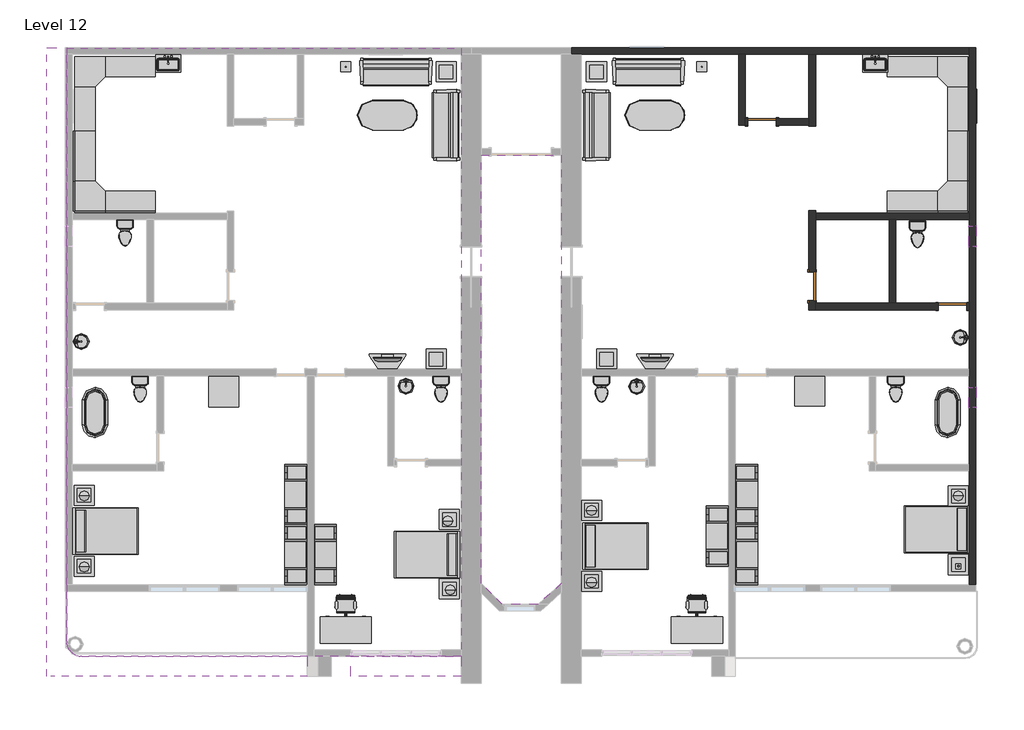
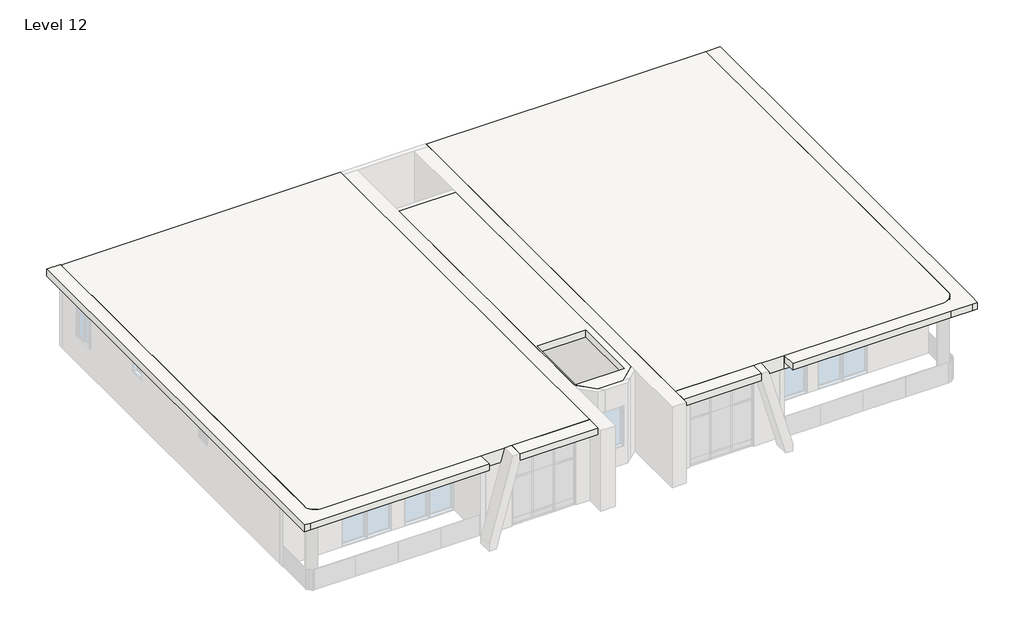
# One storey, part 3 of 3: 42 furniture elements, 14 flow terminals, 10 light fixtures, 9 walls, 4 slabs, 3 doors, 3 windows.
"""IFC4 building model written with IfcOpenShell, lengths in millimetres."""

from ifc_helpers import new_model, si_unit, point, frame, frame_2d, origin, place, context, project, spatial, polyline, circle_curve, trimmed, segment, composite_curve, outline, extrude, faceted_brep, transform, mapped, element, save
from components import door_2703ae13, door_10fd3a06, flow_terminal_38af2918, flow_terminal_d49f872f, toilet_domestic_3d_toilet_domestic_3d_f7549cf7, toilet_domestic_3d_toilet_domestic_3d_183bbd19, flow_terminal_b374fae2, furniture_07436f11, furniture_096e7f55, chair_task_arms_chair_task_arms_fa5a08ef, furniture_072f6425, furniture_cf0b6580, furniture_aff9b2fb, furniture_56245f3a, tv_stand_tv_stand_6ce107e5, furniture_b5c51a22, furniture_2c34a4f9, furniture_4d44e21c, furniture_45e3acac, light_fixture_100w_120v_8564026f, table_lamp_hemispheric_60w_120v_02721d88, window_0038ecf3, window_54100e87

model = new_model("IFC4")

# Units and contexts
model_context = context("Model", 3, world=origin())
ifc_project = project(units=[si_unit("LENGTHUNIT", "METRE", prefix="MILLI")], contexts=[model_context])

# Site, building, storey
site = spatial("IfcSite", under=ifc_project)
building = spatial("IfcBuilding", under=site)
storey = spatial("IfcBuildingStorey", under=building, Name="Level 12", Elevation=40233.6)

# Doors
placement = place(None, origin())
door_shape = door_2703ae13(model_context)
element("IfcDoor", 1, ObjectType="Door-Single-Panel.0001 : 34\" x 80\"", at=placement, inside=storey, context=model_context, shape_type="MappedRepresentation", body=[
    mapped(door_shape, transform((2522.0012296, 9464.0758558, 40233.6), x_axis=(-1.0, 0.0, 0.0), y_axis=(0.0, -1.0, 0.0), z_axis=(0.0, 0.0, 1.0))),
])
door_2_shape = door_10fd3a06(model_context)
element("IfcDoor", 2, ObjectType="Door-Single-Panel.0001 : 34\" x 80\"", at=placement, inside=storey, context=model_context, shape_type="MappedRepresentation", body=[
    mapped(door_2_shape, transform((8313.2012296, 3850.6758558, 40233.6), x_axis=(1.0, 0.0, 0.0), y_axis=(0.0, 1.0, 0.0), z_axis=(0.0, 0.0, 1.0))),
])
element("IfcDoor", 3, ObjectType="Door-Single-Panel.0001 : 34\" x 80\"", at=placement, inside=storey, context=model_context, shape_type="MappedRepresentation", body=[
    mapped(door_2_shape, transform((4046.0012296, 4460.2758558, 40233.6), x_axis=(0.0, -1.0, 0.0), y_axis=(1.0, 0.0, 0.0), z_axis=(0.0, 0.0, 1.0))),
])

# Flow terminals
flow_terminal_shape = flow_terminal_38af2918(model_context)
element("IfcFlowTerminal", 4, ObjectType="Sink Kitchen-Single : 30\" x 21\"", at=placement, inside=storey, context=model_context, shape_type="MappedRepresentation", body=[
    mapped(flow_terminal_shape, transform((-15540.388011, 11239.7304546, 40233.6), x_axis=(1.0, 0.0, 0.0), y_axis=(0.0, 1.0, 0.0), z_axis=(0.0, 0.0, 1.0))),
])
element("IfcFlowTerminal", 5, ObjectType="Sink Kitchen-Single : 30\" x 21\"", at=placement, inside=storey, context=model_context, shape_type="MappedRepresentation", body=[
    mapped(flow_terminal_shape, transform((5948.011989, 11239.7304546, 40233.6), x_axis=(1.0, 0.0, 0.0), y_axis=(0.0, 1.0, 0.0), z_axis=(0.0, 0.0, 1.0))),
])
flow_terminal_2_shape = flow_terminal_d49f872f(model_context)
element("IfcFlowTerminal", 6, ObjectType="Sink Vanity-Round : 19\" x 19\"", at=placement, inside=storey, context=model_context, shape_type="MappedRepresentation", body=[
    mapped(flow_terminal_2_shape, transform((-18084.6070794, 2687.2241152, 40233.6), x_axis=(0.0, 1.0, 0.0), y_axis=(-1.0, 0.0, 0.0), z_axis=(0.0, 0.0, 1.0))),
])
element("IfcFlowTerminal", 7, ObjectType="Sink Vanity-Round : 19\" x 19\"", at=placement, inside=storey, context=model_context, shape_type="MappedRepresentation", body=[
    mapped(flow_terminal_2_shape, transform((8462.2249463, 3007.5275963, 40233.6), x_axis=(0.0, -1.0, 0.0), y_axis=(1.0, 0.0, 0.0), z_axis=(0.0, 0.0, 1.0))),
])
element("IfcFlowTerminal", 8, ObjectType="Sink Vanity-Round : 19\" x 19\"", at=placement, inside=storey, context=model_context, shape_type="MappedRepresentation", body=[
    mapped(flow_terminal_2_shape, transform((-8395.050511, 1341.8921141, 40233.6), x_axis=(1.0, 0.0, 0.0), y_axis=(0.0, 1.0, 0.0), z_axis=(0.0, 0.0, 1.0))),
])
element("IfcFlowTerminal", 9, ObjectType="Sink Vanity-Round : 19\" x 19\"", at=placement, inside=storey, context=model_context, shape_type="MappedRepresentation", body=[
    mapped(flow_terminal_2_shape, transform((-1384.650511, 1331.0855344, 40233.6), x_axis=(1.0, 0.0, 0.0), y_axis=(0.0, 1.0, 0.0), z_axis=(0.0, 0.0, 1.0))),
])
toilet_domestic_3d_toilet_domestic_3d_shape = toilet_domestic_3d_toilet_domestic_3d_f7549cf7(model_context)
toilet_domestic_3d_toilet_domestic_3d_2_shape = toilet_domestic_3d_toilet_domestic_3d_183bbd19(model_context)
element("IfcFlowTerminal", 10, ObjectType="Toilet-Domestic-3D : Toilet-Domestic-3D", at=placement, inside=storey, context=model_context, shape_type="MappedRepresentation", body=[
    mapped(toilet_domestic_3d_toilet_domestic_3d_shape, transform((6586.0012296, 1247.7798284, 40233.6), x_axis=(1.0, 0.0, 0.0), y_axis=(0.0, 1.0, 0.0), z_axis=(0.0, 0.0, 1.0))),
    mapped(toilet_domestic_3d_toilet_domestic_3d_2_shape, transform((6586.0012296, 1247.7798284, 40233.6), x_axis=(1.0, 0.0, 0.0), y_axis=(0.0, 1.0, 0.0), z_axis=(0.0, 0.0, 1.0))),
])
element("IfcFlowTerminal", 11, ObjectType="Toilet-Domestic-3D : Toilet-Domestic-3D", at=placement, inside=storey, context=model_context, shape_type="MappedRepresentation", body=[
    mapped(toilet_domestic_3d_toilet_domestic_3d_shape, transform((-2354.7987704, 1247.7798284, 40233.6), x_axis=(1.0, 0.0, 0.0), y_axis=(0.0, 1.0, 0.0), z_axis=(0.0, 0.0, 1.0))),
    mapped(toilet_domestic_3d_toilet_domestic_3d_2_shape, transform((-2354.7987704, 1247.7798284, 40233.6), x_axis=(1.0, 0.0, 0.0), y_axis=(0.0, 1.0, 0.0), z_axis=(0.0, 0.0, 1.0))),
])
element("IfcFlowTerminal", 12, ObjectType="Toilet-Domestic-3D : Toilet-Domestic-3D", at=placement, inside=storey, context=model_context, shape_type="MappedRepresentation", body=[
    mapped(toilet_domestic_3d_toilet_domestic_3d_shape, transform((-16375.5987704, 1247.7798284, 40233.6), x_axis=(1.0, 0.0, 0.0), y_axis=(0.0, 1.0, 0.0), z_axis=(0.0, 0.0, 1.0))),
    mapped(toilet_domestic_3d_toilet_domestic_3d_2_shape, transform((-16375.5987704, 1247.7798284, 40233.6), x_axis=(1.0, 0.0, 0.0), y_axis=(0.0, 1.0, 0.0), z_axis=(0.0, 0.0, 1.0))),
])
element("IfcFlowTerminal", 13, ObjectType="Toilet-Domestic-3D : Toilet-Domestic-3D", at=placement, inside=storey, context=model_context, shape_type="MappedRepresentation", body=[
    mapped(toilet_domestic_3d_toilet_domestic_3d_shape, transform((-16832.7987704, 5997.5798284, 40233.6), x_axis=(1.0, 0.0, 0.0), y_axis=(0.0, 1.0, 0.0), z_axis=(0.0, 0.0, 1.0))),
    mapped(toilet_domestic_3d_toilet_domestic_3d_2_shape, transform((-16832.7987704, 5997.5798284, 40233.6), x_axis=(1.0, 0.0, 0.0), y_axis=(0.0, 1.0, 0.0), z_axis=(0.0, 0.0, 1.0))),
])
element("IfcFlowTerminal", 14, ObjectType="Toilet-Domestic-3D : Toilet-Domestic-3D", at=placement, inside=storey, context=model_context, shape_type="MappedRepresentation", body=[
    mapped(toilet_domestic_3d_toilet_domestic_3d_shape, transform((7246.4012296, 5946.7798284, 40233.6), x_axis=(1.0, 0.0, 0.0), y_axis=(0.0, 1.0, 0.0), z_axis=(0.0, 0.0, 1.0))),
    mapped(toilet_domestic_3d_toilet_domestic_3d_2_shape, transform((7246.4012296, 5946.7798284, 40233.6), x_axis=(1.0, 0.0, 0.0), y_axis=(0.0, 1.0, 0.0), z_axis=(0.0, 0.0, 1.0))),
])
element("IfcFlowTerminal", 15, ObjectType="Toilet-Domestic-3D : Toilet-Domestic-3D", at=placement, inside=storey, context=model_context, shape_type="MappedRepresentation", body=[
    mapped(toilet_domestic_3d_toilet_domestic_3d_shape, transform((-7231.5987704, 1247.7798284, 40233.6), x_axis=(1.0, 0.0, 0.0), y_axis=(0.0, 1.0, 0.0), z_axis=(0.0, 0.0, 1.0))),
    mapped(toilet_domestic_3d_toilet_domestic_3d_2_shape, transform((-7231.5987704, 1247.7798284, 40233.6), x_axis=(1.0, 0.0, 0.0), y_axis=(0.0, 1.0, 0.0), z_axis=(0.0, 0.0, 1.0))),
])
flow_terminal_3_shape = flow_terminal_b374fae2(model_context)
element("IfcFlowTerminal", 16, ObjectType="Tub-Free Standing-3D : 30\" x 60\"", at=placement, inside=storey, context=model_context, shape_type="MappedRepresentation", body=[
    mapped(flow_terminal_3_shape, transform((-17747.1987704, 624.8758558, 40233.6), x_axis=(1.0, 0.0, 0.0), y_axis=(0.0, 1.0, 0.0), z_axis=(0.0, 0.0, 1.0))),
])
element("IfcFlowTerminal", 17, ObjectType="Tub-Free Standing-3D : 30\" x 60\"", at=placement, inside=storey, context=model_context, shape_type="MappedRepresentation", body=[
    mapped(flow_terminal_3_shape, transform((8160.8012296, 624.8758558, 40233.6), x_axis=(1.0, 0.0, 0.0), y_axis=(0.0, 1.0, 0.0), z_axis=(0.0, 0.0, 1.0))),
])

# Furniture
furniture_shape = furniture_07436f11(model_context)
element("IfcFurniture", 18, ObjectType="96\" x 96\"", at=placement, inside=storey, context=model_context, shape_type="MappedRepresentation", body=[
    mapped(furniture_shape, transform((-18275.8670182, 11991.0988634, 40233.6), x_axis=(1.0, 0.0, 0.0), y_axis=(0.0, 1.0, 0.0), z_axis=(0.0, 0.0, 1.0))),
])
element("IfcFurniture", 19, ObjectType="96\" x 96\"", at=placement, inside=storey, context=model_context, shape_type="MappedRepresentation", body=[
    mapped(furniture_shape, transform((9316.2242372, 11364.3441035, 40233.6), x_axis=(0.0, -1.0, 0.0), y_axis=(1.0, 0.0, 0.0), z_axis=(0.0, 0.0, 1.0))),
])
furniture_2_shape = furniture_096e7f55(model_context)
element("IfcFurniture", 20, ObjectType="Bed-Shaker : Double 56\" x 78\"", at=placement, inside=storey, context=model_context, shape_type="MappedRepresentation", body=[
    mapped(furniture_2_shape, transform((-18407.5987704, -2962.8741442, 40233.6), x_axis=(0.0, 1.0, 0.0), y_axis=(-1.0, 0.0, 0.0), z_axis=(0.0, 0.0, 1.0))),
])
element("IfcFurniture", 21, ObjectType="Bed-Shaker : Double 56\" x 78\"", at=placement, inside=storey, context=model_context, shape_type="MappedRepresentation", body=[
    mapped(furniture_2_shape, transform((-6672.7987704, -3712.1741442, 40233.6), x_axis=(0.0, -1.0, 0.0), y_axis=(1.0, 0.0, 0.0), z_axis=(0.0, 0.0, 1.0))),
])
element("IfcFurniture", 22, ObjectType="Bed-Shaker : Double 56\" x 78\"", at=placement, inside=storey, context=model_context, shape_type="MappedRepresentation", body=[
    mapped(furniture_2_shape, transform((-2913.5987704, -3420.0741442, 40233.6), x_axis=(0.0, 1.0, 0.0), y_axis=(-1.0, 0.0, 0.0), z_axis=(0.0, 0.0, 1.0))),
])
element("IfcFurniture", 23, ObjectType="Bed-Shaker : Double 56\" x 78\"", at=placement, inside=storey, context=model_context, shape_type="MappedRepresentation", body=[
    mapped(furniture_2_shape, transform((8821.2012296, -2950.1741442, 40233.6), x_axis=(0.0, -1.0, 0.0), y_axis=(1.0, 0.0, 0.0), z_axis=(0.0, 0.0, 1.0))),
])
chair_task_arms_chair_task_arms_shape = chair_task_arms_chair_task_arms_fa5a08ef(model_context)
element("IfcFurniture", 24, ObjectType="Chair-Task Arms : Chair-Task Arms", at=placement, inside=storey, context=model_context, shape_type="MappedRepresentation", body=[
    mapped(chair_task_arms_chair_task_arms_shape, transform((681.7920493, -5184.3566833, 40233.6), x_axis=(-1.0, 0.0, 0.0), y_axis=(0.0, -1.0, 0.0), z_axis=(0.0, 0.0, 1.0))),
])
element("IfcFurniture", 25, ObjectType="Chair-Task Arms : Chair-Task Arms", at=placement, inside=storey, context=model_context, shape_type="MappedRepresentation", body=[
    mapped(chair_task_arms_chair_task_arms_shape, transform((-9986.2079507, -5184.3566833, 40233.6), x_axis=(-1.0, 0.0, 0.0), y_axis=(0.0, -1.0, 0.0), z_axis=(0.0, 0.0, 1.0))),
])
furniture_3_shape = furniture_072f6425(model_context)
element("IfcFurniture", 26, ObjectType="Desk : 60\" x 30\"", at=placement, inside=storey, context=model_context, shape_type="MappedRepresentation", body=[
    mapped(furniture_3_shape, transform((-10889.1987704, -6371.702585, 40233.6), x_axis=(1.0, 0.0, 0.0), y_axis=(0.0, 1.0, 0.0), z_axis=(0.0, 0.0, 1.0))),
])
element("IfcFurniture", 27, ObjectType="Desk : 60\" x 30\"", at=placement, inside=storey, context=model_context, shape_type="MappedRepresentation", body=[
    mapped(furniture_3_shape, transform((-221.1987704, -6371.702585, 40233.6), x_axis=(1.0, 0.0, 0.0), y_axis=(0.0, 1.0, 0.0), z_axis=(0.0, 0.0, 1.0))),
])
furniture_4_shape = furniture_cf0b6580(model_context)
element("IfcFurniture", 28, ObjectType="Entertainment Center : 72\" x 72\" x 24\"", at=placement, inside=storey, context=model_context, shape_type="MappedRepresentation", body=[
    mapped(furniture_4_shape, transform((1607.6012296, -3134.3241442, 40233.6), x_axis=(0.0, -1.0, 0.0), y_axis=(1.0, 0.0, 0.0), z_axis=(0.0, 0.0, 1.0))),
])
element("IfcFurniture", 29, ObjectType="Entertainment Center : 72\" x 72\" x 24\"", at=placement, inside=storey, context=model_context, shape_type="MappedRepresentation", body=[
    mapped(furniture_4_shape, transform((1607.6012296, -3693.1241442, 40233.6), x_axis=(0.0, 1.0, 0.0), y_axis=(-1.0, 0.0, 0.0), z_axis=(0.0, 0.0, 1.0))),
])
element("IfcFurniture", 30, ObjectType="Entertainment Center : 72\" x 72\" x 24\"", at=placement, inside=storey, context=model_context, shape_type="MappedRepresentation", body=[
    mapped(furniture_4_shape, transform((1607.6012296, -1864.3241442, 40233.6), x_axis=(0.0, 1.0, 0.0), y_axis=(-1.0, 0.0, 0.0), z_axis=(0.0, 0.0, 1.0))),
])
element("IfcFurniture", 31, ObjectType="Entertainment Center : 72\" x 72\" x 24\"", at=placement, inside=storey, context=model_context, shape_type="MappedRepresentation", body=[
    mapped(furniture_4_shape, transform((-11193.9987704, -3693.1241442, 40233.6), x_axis=(0.0, -1.0, 0.0), y_axis=(1.0, 0.0, 0.0), z_axis=(0.0, 0.0, 1.0))),
])
element("IfcFurniture", 32, ObjectType="Entertainment Center : 72\" x 72\" x 24\"", at=placement, inside=storey, context=model_context, shape_type="MappedRepresentation", body=[
    mapped(furniture_4_shape, transform((-11193.9987704, -1864.3241442, 40233.6), x_axis=(0.0, -1.0, 0.0), y_axis=(1.0, 0.0, 0.0), z_axis=(0.0, 0.0, 1.0))),
])
element("IfcFurniture", 33, ObjectType="Entertainment Center : 72\" x 72\" x 24\"", at=placement, inside=storey, context=model_context, shape_type="MappedRepresentation", body=[
    mapped(furniture_4_shape, transform((-11193.9987704, -3693.1241442, 40233.6), x_axis=(0.0, 1.0, 0.0), y_axis=(-1.0, 0.0, 0.0), z_axis=(0.0, 0.0, 1.0))),
])
furniture_5_shape = furniture_aff9b2fb(model_context)
element("IfcFurniture", 34, ObjectType="Sofa-Pensi : 84\"", at=placement, inside=storey, context=model_context, shape_type="MappedRepresentation", body=[
    mapped(furniture_5_shape, transform((-8881.8050204, 10710.9660197, 40233.6), x_axis=(1.0, 0.0, 0.0), y_axis=(0.0, 1.0, 0.0), z_axis=(0.0, 0.0, 1.0))),
])
element("IfcFurniture", 35, ObjectType="Sofa-Pensi : 84\"", at=placement, inside=storey, context=model_context, shape_type="MappedRepresentation", body=[
    mapped(furniture_5_shape, transform((-7356.3086065, 9641.0821058, 40233.6), x_axis=(0.0, -1.0, 0.0), y_axis=(1.0, 0.0, 0.0), z_axis=(0.0, 0.0, 1.0))),
])
element("IfcFurniture", 36, ObjectType="Sofa-Pensi : 84\"", at=placement, inside=storey, context=model_context, shape_type="MappedRepresentation", body=[
    mapped(furniture_5_shape, transform((-2230.0889343, 9083.8696058, 40233.6), x_axis=(0.0, 1.0, 0.0), y_axis=(-1.0, 0.0, 0.0), z_axis=(0.0, 0.0, 1.0))),
])
element("IfcFurniture", 37, ObjectType="Sofa-Pensi : 84\"", at=placement, inside=storey, context=model_context, shape_type="MappedRepresentation", body=[
    mapped(furniture_5_shape, transform((-1211.0050204, 10710.9660197, 40233.6), x_axis=(1.0, 0.0, 0.0), y_axis=(0.0, 1.0, 0.0), z_axis=(0.0, 0.0, 1.0))),
])
furniture_6_shape = furniture_56245f3a(model_context)
element("IfcFurniture", 38, ObjectType="TV - Flat Screen : 32\"", at=placement, inside=storey, context=model_context, shape_type="MappedRepresentation", body=[
    mapped(furniture_6_shape, transform((-8861.1432846, 2232.8144794, 41148.0), x_axis=(-1.0, 0.0, 0.0), y_axis=(0.0, -1.0, 0.0), z_axis=(0.0, 0.0, 1.0))),
])
element("IfcFurniture", 39, ObjectType="TV - Flat Screen : 32\"", at=placement, inside=storey, context=model_context, shape_type="MappedRepresentation", body=[
    mapped(furniture_6_shape, transform((-733.1432846, 2232.8144794, 41148.0), x_axis=(-1.0, 0.0, 0.0), y_axis=(0.0, -1.0, 0.0), z_axis=(0.0, 0.0, 1.0))),
])
tv_stand_tv_stand_shape = tv_stand_tv_stand_6ce107e5(model_context)
element("IfcFurniture", 40, ObjectType="TV Stand : TV Stand", at=placement, inside=storey, context=model_context, shape_type="MappedRepresentation", body=[
    mapped(tv_stand_tv_stand_shape, transform((-8732.0107683, 1945.6758558, 40233.6), x_axis=(-1.0, 0.0, 0.0), y_axis=(0.0, -1.0, 0.0), z_axis=(0.0, 0.0, 1.0))),
])
element("IfcFurniture", 41, ObjectType="TV Stand : TV Stand", at=placement, inside=storey, context=model_context, shape_type="MappedRepresentation", body=[
    mapped(tv_stand_tv_stand_shape, transform((-604.0107683, 1945.6758558, 40233.6), x_axis=(-1.0, 0.0, 0.0), y_axis=(0.0, -1.0, 0.0), z_axis=(0.0, 0.0, 1.0))),
])
furniture_7_shape = furniture_b5c51a22(model_context)
element("IfcFurniture", 42, ObjectType="Table-Coffee : 24\" x 24\" x 24\"", at=placement, inside=storey, context=model_context, shape_type="MappedRepresentation", body=[
    mapped(furniture_7_shape, transform((-7097.4645371, 10892.864778, 40233.6), x_axis=(1.0, 0.0, 0.0), y_axis=(0.0, 1.0, 0.0), z_axis=(0.0, 0.0, 1.0))),
])
element("IfcFurniture", 43, ObjectType="Table-Coffee : 24\" x 24\" x 24\"", at=placement, inside=storey, context=model_context, shape_type="MappedRepresentation", body=[
    mapped(furniture_7_shape, transform((-2525.4645371, 10892.864778, 40233.6), x_axis=(1.0, 0.0, 0.0), y_axis=(0.0, 1.0, 0.0), z_axis=(0.0, 0.0, 1.0))),
])
element("IfcFurniture", 44, ObjectType="Table-Coffee : 24\" x 24\" x 24\"", at=placement, inside=storey, context=model_context, shape_type="MappedRepresentation", body=[
    mapped(furniture_7_shape, transform((-7402.2645371, 2155.264778, 40233.6), x_axis=(1.0, 0.0, 0.0), y_axis=(0.0, 1.0, 0.0), z_axis=(0.0, 0.0, 1.0))),
])
element("IfcFurniture", 45, ObjectType="Table-Coffee : 24\" x 24\" x 24\"", at=placement, inside=storey, context=model_context, shape_type="MappedRepresentation", body=[
    mapped(furniture_7_shape, transform((-2220.6645371, 2155.264778, 40233.6), x_axis=(1.0, 0.0, 0.0), y_axis=(0.0, 1.0, 0.0), z_axis=(0.0, 0.0, 1.0))),
])
element("IfcFurniture", 46, ObjectType="Table-Coffee : 24\" x 24\" x 24\"", at=placement, inside=storey, context=model_context, shape_type="MappedRepresentation", body=[
    mapped(furniture_7_shape, transform((-2677.8645371, -4601.135222, 40233.6), x_axis=(1.0, 0.0, 0.0), y_axis=(0.0, 1.0, 0.0), z_axis=(0.0, 0.0, 1.0))),
])
element("IfcFurniture", 47, ObjectType="Table-Coffee : 24\" x 24\" x 24\"", at=placement, inside=storey, context=model_context, shape_type="MappedRepresentation", body=[
    mapped(furniture_7_shape, transform((-18095.6645371, -4143.935222, 40233.6), x_axis=(1.0, 0.0, 0.0), y_axis=(0.0, 1.0, 0.0), z_axis=(0.0, 0.0, 1.0))),
])
element("IfcFurniture", 48, ObjectType="Table-Coffee : 24\" x 24\" x 24\"", at=placement, inside=storey, context=model_context, shape_type="MappedRepresentation", body=[
    mapped(furniture_7_shape, transform((-18095.6645371, -1984.935222, 40233.6), x_axis=(1.0, 0.0, 0.0), y_axis=(0.0, 1.0, 0.0), z_axis=(0.0, 0.0, 1.0))),
])
element("IfcFurniture", 49, ObjectType="Table-Coffee : 24\" x 24\" x 24\"", at=placement, inside=storey, context=model_context, shape_type="MappedRepresentation", body=[
    mapped(furniture_7_shape, transform((-2677.8645371, -2442.135222, 40233.6), x_axis=(1.0, 0.0, 0.0), y_axis=(0.0, 1.0, 0.0), z_axis=(0.0, 0.0, 1.0))),
])
element("IfcFurniture", 50, ObjectType="Table-Coffee : 24\" x 24\" x 24\"", at=placement, inside=storey, context=model_context, shape_type="MappedRepresentation", body=[
    mapped(furniture_7_shape, transform((8472.7354629, -4093.135222, 40233.6), x_axis=(1.0, 0.0, 0.0), y_axis=(0.0, 1.0, 0.0), z_axis=(0.0, 0.0, 1.0))),
])
element("IfcFurniture", 51, ObjectType="Table-Coffee : 24\" x 24\" x 24\"", at=placement, inside=storey, context=model_context, shape_type="MappedRepresentation", body=[
    mapped(furniture_7_shape, transform((8472.7354629, -2010.335222, 40233.6), x_axis=(1.0, 0.0, 0.0), y_axis=(0.0, 1.0, 0.0), z_axis=(0.0, 0.0, 1.0))),
])
element("IfcFurniture", 52, ObjectType="Table-Coffee : 24\" x 24\" x 24\"", at=placement, inside=storey, context=model_context, shape_type="MappedRepresentation", body=[
    mapped(furniture_7_shape, transform((-6995.8645371, -4832.0414601, 40233.6), x_axis=(1.0, 0.0, 0.0), y_axis=(0.0, 1.0, 0.0), z_axis=(0.0, 0.0, 1.0))),
])
element("IfcFurniture", 53, ObjectType="Table-Coffee : 24\" x 24\" x 24\"", at=placement, inside=storey, context=model_context, shape_type="MappedRepresentation", body=[
    mapped(furniture_7_shape, transform((-6995.8645371, -2723.8414601, 40233.6), x_axis=(1.0, 0.0, 0.0), y_axis=(0.0, 1.0, 0.0), z_axis=(0.0, 0.0, 1.0))),
])
furniture_8_shape = furniture_2c34a4f9(model_context)
element("IfcFurniture", 54, ObjectType="Table-Dining Oval : 36\" x 72\"", at=placement, inside=storey, context=model_context, shape_type="MappedRepresentation", body=[
    mapped(furniture_8_shape, transform((-8455.3790983, 10025.3742164, 40233.6), x_axis=(1.0, 0.0, 0.0), y_axis=(0.0, 1.0, 0.0), z_axis=(0.0, 0.0, 1.0))),
])
element("IfcFurniture", 55, ObjectType="Table-Dining Oval : 36\" x 72\"", at=placement, inside=storey, context=model_context, shape_type="MappedRepresentation", body=[
    mapped(furniture_8_shape, transform((-327.3790983, 10025.3742164, 40233.6), x_axis=(1.0, 0.0, 0.0), y_axis=(0.0, 1.0, 0.0), z_axis=(0.0, 0.0, 1.0))),
])
furniture_9_shape = furniture_4d44e21c(model_context)
element("IfcFurniture", 56, ObjectType="Table-Rectangular : 36\" x 36\"", at=placement, inside=storey, context=model_context, shape_type="MappedRepresentation", body=[
    mapped(furniture_9_shape, transform((-13835.5987704, 1259.8758558, 40233.6), x_axis=(1.0, 0.0, 0.0), y_axis=(0.0, 1.0, 0.0), z_axis=(0.0, 0.0, 1.0))),
])
element("IfcFurniture", 57, ObjectType="Table-Rectangular : 36\" x 36\"", at=placement, inside=storey, context=model_context, shape_type="MappedRepresentation", body=[
    mapped(furniture_9_shape, transform((3969.8012296, 1285.2758558, 40233.6), x_axis=(1.0, 0.0, 0.0), y_axis=(0.0, 1.0, 0.0), z_axis=(0.0, 0.0, 1.0))),
])
furniture_10_shape = furniture_45e3acac(model_context)
element("IfcFurniture", 58, ObjectType="Work Station Cubicle : 96\" x 96\"", at=placement, inside=storey, context=model_context, shape_type="MappedRepresentation", body=[
    mapped(furniture_10_shape, transform((-18902.621778, 6827.207608, 40233.6), x_axis=(0.0, 1.0, 0.0), y_axis=(-1.0, 0.0, 0.0), z_axis=(0.0, 0.0, 1.0))),
])
element("IfcFurniture", 59, ObjectType="Work Station Cubicle : 96\" x 96\"", at=placement, inside=storey, context=model_context, shape_type="MappedRepresentation", body=[
    mapped(furniture_10_shape, transform((8689.4694774, 6200.4528481, 40233.6), x_axis=(-1.0, 0.0, 0.0), y_axis=(0.0, -1.0, 0.0), z_axis=(0.0, 0.0, 1.0))),
])

# Light fixtures
light_fixture_100w_120v_shape = light_fixture_100w_120v_8564026f(model_context)
element("IfcLightFixture", 60, ObjectType="100W - 120V", at=placement, inside=storey, context=model_context, shape_type="MappedRepresentation", body=[
    mapped(light_fixture_100w_120v_shape, transform((-10127.1987704, 11140.4758558, 40233.6), x_axis=(1.0, 0.0, 0.0), y_axis=(0.0, 1.0, 0.0), z_axis=(0.0, 0.0, 1.0))),
])
element("IfcLightFixture", 61, ObjectType="100W - 120V", at=placement, inside=storey, context=model_context, shape_type="MappedRepresentation", body=[
    mapped(light_fixture_100w_120v_shape, transform((693.2012296, 11140.4758558, 40233.6), x_axis=(1.0, 0.0, 0.0), y_axis=(0.0, 1.0, 0.0), z_axis=(0.0, 0.0, 1.0))),
])
table_lamp_hemispheric_60w_120v_shape = table_lamp_hemispheric_60w_120v_02721d88(model_context)
element("IfcLightFixture", 62, ObjectType="Table Lamp - Hemispheric : 60W - 120V", at=placement, inside=storey, context=model_context, shape_type="MappedRepresentation", body=[
    mapped(table_lamp_hemispheric_60w_120v_shape, transform((-18077.3987704, -1915.1241442, 40843.2), x_axis=(1.0, 0.0, 0.0), y_axis=(0.0, 1.0, 0.0), z_axis=(0.0, 0.0, 1.0))),
])
element("IfcLightFixture", 63, ObjectType="Table Lamp - Hemispheric : 60W - 120V", at=placement, inside=storey, context=model_context, shape_type="MappedRepresentation", body=[
    mapped(table_lamp_hemispheric_60w_120v_shape, transform((-7028.3987704, -2666.7303823, 40843.2), x_axis=(1.0, 0.0, 0.0), y_axis=(0.0, 1.0, 0.0), z_axis=(0.0, 0.0, 1.0))),
])
element("IfcLightFixture", 64, ObjectType="Table Lamp - Hemispheric : 60W - 120V", at=placement, inside=storey, context=model_context, shape_type="MappedRepresentation", body=[
    mapped(table_lamp_hemispheric_60w_120v_shape, transform((-2659.5987704, -2346.9241442, 40843.2), x_axis=(1.0, 0.0, 0.0), y_axis=(0.0, 1.0, 0.0), z_axis=(0.0, 0.0, 1.0))),
])
element("IfcLightFixture", 65, ObjectType="Table Lamp - Hemispheric : 60W - 120V", at=placement, inside=storey, context=model_context, shape_type="MappedRepresentation", body=[
    mapped(table_lamp_hemispheric_60w_120v_shape, transform((8491.0012296, -4048.7241442, 41148.0), x_axis=(1.0, 0.0, 0.0), y_axis=(0.0, 1.0, 0.0), z_axis=(0.0, 0.0, 1.0))),
])
element("IfcLightFixture", 66, ObjectType="Table Lamp - Hemispheric : 60W - 120V", at=placement, inside=storey, context=model_context, shape_type="MappedRepresentation", body=[
    mapped(table_lamp_hemispheric_60w_120v_shape, transform((8491.0012296, -1915.1241442, 40843.2), x_axis=(1.0, 0.0, 0.0), y_axis=(0.0, 1.0, 0.0), z_axis=(0.0, 0.0, 1.0))),
])
element("IfcLightFixture", 67, ObjectType="Table Lamp - Hemispheric : 60W - 120V", at=placement, inside=storey, context=model_context, shape_type="MappedRepresentation", body=[
    mapped(table_lamp_hemispheric_60w_120v_shape, transform((-2659.5987704, -4531.3241442, 40843.2), x_axis=(1.0, 0.0, 0.0), y_axis=(0.0, 1.0, 0.0), z_axis=(0.0, 0.0, 1.0))),
])
element("IfcLightFixture", 68, ObjectType="Table Lamp - Hemispheric : 60W - 120V", at=placement, inside=storey, context=model_context, shape_type="MappedRepresentation", body=[
    mapped(table_lamp_hemispheric_60w_120v_shape, transform((-6952.1987704, -4762.2303823, 40843.2), x_axis=(1.0, 0.0, 0.0), y_axis=(0.0, 1.0, 0.0), z_axis=(0.0, 0.0, 1.0))),
])
element("IfcLightFixture", 69, ObjectType="Table Lamp - Hemispheric : 60W - 120V", at=placement, inside=storey, context=model_context, shape_type="MappedRepresentation", body=[
    mapped(table_lamp_hemispheric_60w_120v_shape, transform((-18077.3987704, -4074.1241442, 40843.2), x_axis=(1.0, 0.0, 0.0), y_axis=(0.0, 1.0, 0.0), z_axis=(0.0, 0.0, 1.0))),
])

# Slabs
element("IfcSlab", 70, ObjectType="Generic - 12\" cream", at=placement, inside=storey, context=model_context, shape_type="SweptSolid", body=[
    extrude(outline(composite_curve([segment(polyline([(-6621.9987704, 11699.2758558), (-6621.9987704, -6791.9241442), (-11295.5987704, -6791.9241442), (-18153.5987704, -6791.9241442)]), True, "CONTINUOUS"), segment(trimmed(circle_curve(frame_2d((-18153.5987704, -6334.7241442)), 457.2), [point((-18153.5987704, -6791.9241442))], [point((-18610.7987704, -6334.7241442))], False, "CARTESIAN"), True, "CONTINUOUS"), segment(polyline([(-18610.7987704, -6334.7241442), (-18610.7987704, 11699.2758558), (-6621.9987704, 11699.2758558)]), True, "CONTINUOUS")], self_intersect=False)), frame((0.0, 0.0, 43281.6), z_axis=(0.0, 0.0, 1.0), x_axis=(1.0, 0.0, 0.0)), (0.0, 0.0, 1.0), 609.6),
    extrude(outline(composite_curve([segment(trimmed(circle_curve(frame_2d((8511.8043381, -6277.3874522)), 514.536692), [point((9024.4012296, -6322.0241442))], [point((8511.8043381, -6791.9241442))], False, "CARTESIAN"), True, "CONTINUOUS"), segment(polyline([(8511.8043381, -6791.9241442), (1709.2012296, -6791.9241442), (-2862.7987704, -6791.9241442), (-2964.3987704, -6791.9241442), (-2964.3987704, 11699.2758558), (9024.4012296, 11699.2758558), (9024.4012296, -6322.0241442)]), True, "CONTINUOUS")], self_intersect=False)), frame((0.0, 0.0, 43281.6), z_axis=(0.0, 0.0, 1.0), x_axis=(1.0, 0.0, 0.0)), (0.0, 0.0, 1.0), 609.6),
])
element("IfcSlab", 71, ObjectType="Generic - 12\" white", at=placement, inside=storey, context=model_context, shape_type="SweptSolid", body=[
    extrude(outline(composite_curve([segment(polyline([(9634.0012296, 11699.2758558), (9634.0012296, -6931.6241442), (9634.0012296, -7401.5241442), (9430.8012296, -7401.5241442), (8511.8043381, -7401.5241442), (1709.2012296, -7401.5241442), (1709.2012296, -6791.9241442), (8511.8043381, -6791.9241442)]), True, "CONTINUOUS"), segment(trimmed(circle_curve(frame_2d((8511.8043381, -6277.3874522)), 514.536692), [point((8511.8043381, -6791.9241442))], [point((9024.4012296, -6322.0241442))], True, "CARTESIAN"), True, "CONTINUOUS"), segment(polyline([(9024.4012296, -6322.0241442), (9024.4012296, 11699.2758558), (9634.0012296, 11699.2758558)]), True, "CONTINUOUS")], self_intersect=False)), frame((0.0, 0.0, 43586.4), z_axis=(0.0, 0.0, 1.0), x_axis=(1.0, 0.0, 0.0)), (0.0, 0.0, 1.0), 304.8),
    extrude(outline(composite_curve([segment(polyline([(-18610.7987704, 11724.6758558), (-18610.7987704, -6334.7241442)]), True, "CONTINUOUS"), segment(trimmed(circle_curve(frame_2d((-18153.5987704, -6334.7241442)), 457.2), [point((-18610.7987704, -6334.7241442))], [point((-18153.5987704, -6791.9241442))], True, "CARTESIAN"), True, "CONTINUOUS"), segment(polyline([(-18153.5987704, -6791.9241442), (-11295.5987704, -6791.9241442), (-11295.5987704, -7401.5241442), (-18966.3987704, -7401.5241442), (-19220.3987704, -7401.5241442), (-19220.3987704, 11724.6758558), (-18610.7987704, 11724.6758558)]), True, "CONTINUOUS")], self_intersect=False)), frame((0.0, 0.0, 43586.4), z_axis=(0.0, 0.0, 1.0), x_axis=(1.0, 0.0, 0.0)), (0.0, 0.0, 1.0), 304.8),
])
element("IfcSlab", 72, ObjectType="Generic - 12\" white", at=placement, inside=storey, context=model_context, shape_type="SweptSolid", body=[
    extrude(outline(polyline([(394.7512296, -6791.9241442), (394.7512296, -7401.5241442), (-2958.0487704, -7401.5241442), (-2958.0487704, -6791.9241442), (394.7512296, -6791.9241442)])), frame((0.0, 0.0, 43586.4), z_axis=(0.0, 0.0, 1.0), x_axis=(1.0, 0.0, 0.0)), (0.0, 0.0, 1.0), 304.8),
    extrude(outline(polyline([(-9974.7987704, -6791.9241442), (-6621.9987704, -6791.9241442), (-6621.9987704, -7401.5241442), (-9974.7987704, -7401.5241442), (-9974.7987704, -6791.9241442)])), frame((0.0, 0.0, 43586.4), z_axis=(0.0, 0.0, 1.0), x_axis=(1.0, 0.0, 0.0)), (0.0, 0.0, 1.0), 304.8),
])
element("IfcSlab", 73, ObjectType="Generic - 12\" white", at=placement, inside=storey, context=model_context, shape_type="SweptSolid", body=[
    extrude(outline(polyline([(-3573.9987704, 8448.0758558), (-3573.9987704, -1691.5549149), (-3573.9987704, -4572.9908503), (-4280.7801413, -5203.302585), (-5374.5362318, -5203.302585), (-6012.3987704, -4565.4400463), (-6012.3987704, -1691.5549149), (-6012.3987704, 8448.0758558), (-3573.9987704, 8448.0758558)]), holes=[polyline([(-5940.8822214, -4528.8130548), (-5940.8822214, -4561.7549149), (-3858.0822214, -4561.7549149), (-3858.0822214, -1691.5549149), (-5940.8822214, -1691.5549149), (-5940.8822214, -4528.8130548)])]), frame((0.0, 0.0, 43586.4), z_axis=(0.0, 0.0, 1.0), x_axis=(1.0, 0.0, 0.0)), (0.0, 0.0, 1.0), 304.8),
])

# Walls
element("IfcWall", 74, ObjectType="Generic - 8\" cream", at=placement, inside=storey, context=model_context, shape_type="Brep", body=[
    faceted_brep([(8821.2012296, 11724.6758558, 40233.6), (8821.2012296, 11521.4758558, 40233.6), (8821.2012296, 6695.4758558, 40233.6), (8821.2012296, 6492.2758558, 40233.6), (8821.2012296, 3952.2758558, 40233.6), (8821.2012296, 3749.0758558, 40233.6), (8821.2012296, 1945.6758558, 40233.6), (8821.2012296, 1742.4758558, 40233.6), (8821.2012296, -949.9241442, 40233.6), (8821.2012296, -1153.1241442, 40233.6), (8821.2012296, -4607.5241442, 40233.6), (8821.2012296, -4607.5241442, 43281.6), (8821.2012296, -1153.1241442, 43281.6), (8821.2012296, -949.9241442, 43281.6), (8821.2012296, 1742.4758558, 43281.6), (8821.2012296, 1945.6758558, 43281.6), (8821.2012296, 3749.0758558, 43281.6), (8821.2012296, 3952.2758558, 43281.6), (8821.2012296, 6492.2758558, 43281.6), (8821.2012296, 6695.4758558, 43281.6), (8821.2012296, 11521.4758558, 43281.6), (8821.2012296, 11724.6758558, 43281.6), (8821.2012296, 10403.8758558, 41452.8), (8821.2012296, 10403.8758558, 42672.0), (8821.2012296, 9489.4758558, 42672.0), (8821.2012296, 9489.4758558, 41452.8), (8821.2012296, 777.2758558, 42976.8), (8821.2012296, 777.2758558, 42367.2), (8821.2012296, 1386.8758558, 42367.2), (8821.2012296, 1386.8758558, 42976.8), (8821.2012296, 6289.0758558, 42367.2), (8821.2012296, 6289.0758558, 42976.8), (8821.2012296, 5679.4758558, 42976.8), (8821.2012296, 5679.4758558, 42367.2), (9024.4012296, -4607.5241442, 40233.6), (9024.4012296, 11724.6758558, 40233.6), (9024.4012296, 11724.6758558, 43281.6), (9024.4012296, -4607.5241442, 43281.6), (9024.4012296, 10403.8758558, 42672.0), (9024.4012296, 10403.8758558, 41452.8), (9024.4012296, 9489.4758558, 41452.8), (9024.4012296, 9489.4758558, 42672.0), (9024.4012296, 777.2758558, 42367.2), (9024.4012296, 777.2758558, 42976.8), (9024.4012296, 1386.8758558, 42976.8), (9024.4012296, 1386.8758558, 42367.2), (9024.4012296, 6289.0758558, 42976.8), (9024.4012296, 6289.0758558, 42367.2), (9024.4012296, 5679.4758558, 42367.2), (9024.4012296, 5679.4758558, 42976.8)], [[[0, 1, 2, 3, 4, 5, 6, 7, 8, 9, 10, 11, 12, 13, 14, 15, 16, 17, 18, 19, 20, 21], [22, 23, 24, 25], [26, 27, 28, 29], [30, 31, 32, 33]], [[34, 35, 36, 37], [38, 39, 40, 41], [42, 43, 44, 45], [46, 47, 48, 49]], [[10, 9, 8, 7, 6, 5, 4, 3, 2, 1, 0, 35, 34]], [[21, 20, 19, 18, 17, 16, 15, 14, 13, 12, 11, 37, 36]], [[0, 21, 36, 35]], [[11, 10, 34, 37]], [[39, 38, 23, 22]], [[40, 39, 22, 25]], [[41, 40, 25, 24]], [[38, 41, 24, 23]], [[26, 43, 42, 27]], [[27, 42, 45, 28]], [[28, 45, 44, 29]], [[43, 26, 29, 44]], [[46, 31, 30, 47]], [[47, 30, 33, 48]], [[48, 33, 32, 49]], [[31, 46, 49, 32]]]),
])
element("IfcWall", 75, ObjectType="Generic - 8\" cream", at=placement, inside=storey, context=model_context, shape_type="Brep", body=[
    faceted_brep([(3944.4012296, 11521.4758558, 40233.6), (3944.4012296, 9565.6758558, 40233.6), (3944.4012296, 9362.4758558, 40233.6), (3944.4012296, 9337.0758558, 40233.6), (3944.4012296, 9337.0758558, 43281.6), (3944.4012296, 9362.4758558, 43281.6), (3944.4012296, 9565.6758558, 43281.6), (3944.4012296, 11521.4758558, 43281.6), (4147.6012296, 11521.4758558, 40233.6), (4147.6012296, 11521.4758558, 43281.6), (4147.6012296, 9337.0758558, 43281.6), (4147.6012296, 9337.0758558, 40233.6)], [[[0, 1, 2, 3, 4, 5, 6, 7]], [[8, 9, 10, 11]], [[3, 2, 1, 0, 8, 11]], [[4, 3, 11, 10]], [[7, 6, 5, 4, 10, 9]], [[0, 7, 9, 8]]]),
])
element("IfcWall", 76, ObjectType="Generic - 8\" cream", at=placement, inside=storey, context=model_context, shape_type="Brep", body=[
    faceted_brep([(4147.6012296, 6492.2758558, 40233.6), (6382.8012296, 6492.2758558, 40233.6), (6586.0012296, 6492.2758558, 40233.6), (8821.2012296, 6492.2758558, 40233.6), (8821.2012296, 6492.2758558, 43281.6), (6586.0012296, 6492.2758558, 43281.6), (6382.8012296, 6492.2758558, 43281.6), (4147.6012296, 6492.2758558, 43281.6), (4147.6012296, 6695.4758558, 40233.6), (4147.6012296, 6695.4758558, 43281.6), (8821.2012296, 6695.4758558, 43281.6), (8821.2012296, 6695.4758558, 40233.6)], [[[0, 1, 2, 3, 4, 5, 6, 7]], [[8, 9, 10, 11]], [[3, 2, 1, 0, 8, 11]], [[7, 6, 5, 4, 10, 9]], [[0, 7, 9, 8]], [[4, 3, 11, 10]]]),
])
element("IfcWall", 77, ObjectType="Generic - 8\" cream", at=placement, inside=storey, context=model_context, shape_type="Brep", body=[
    faceted_brep([(8821.2012296, 3749.0758558, 43281.6), (4147.6012296, 3749.0758558, 43281.6), (4147.6012296, 3749.0758558, 40233.6), (7881.4012296, 3749.0758558, 40233.6), (7881.4012296, 3749.0758558, 42265.6), (8745.0012296, 3749.0758558, 42265.6), (8745.0012296, 3749.0758558, 40233.6), (8821.2012296, 3749.0758558, 40233.6), (4147.6012296, 3952.2758558, 43281.6), (6382.8012296, 3952.2758558, 43281.6), (6586.0012296, 3952.2758558, 43281.6), (8821.2012296, 3952.2758558, 43281.6), (8821.2012296, 3952.2758558, 40233.6), (8745.0012296, 3952.2758558, 40233.6), (8745.0012296, 3952.2758558, 42265.6), (7881.4012296, 3952.2758558, 42265.6), (7881.4012296, 3952.2758558, 40233.6), (6586.0012296, 3952.2758558, 40233.6), (6382.8012296, 3952.2758558, 40233.6), (4147.6012296, 3952.2758558, 40233.6)], [[[0, 1, 2, 3, 4, 5, 6, 7]], [[8, 9, 10, 11, 12, 13, 14, 15, 16, 17, 18, 19]], [[2, 19, 18, 17, 16, 3]], [[12, 7, 6, 13]], [[1, 0, 11, 10, 9, 8]], [[2, 1, 8, 19]], [[0, 7, 12, 11]], [[5, 14, 13, 6]], [[14, 5, 4, 15]], [[15, 4, 3, 16]]]),
])
element("IfcWall", 78, ObjectType="Generic - 8\" cream", at=placement, inside=storey, context=model_context, shape_type="SweptSolid", body=[
    extrude(outline(polyline([(43281.6, 3944.4012296), (43281.6, 2014.0012296), (40233.6, 2014.0012296), (40233.6, 2090.2012296), (42265.6, 2090.2012296), (42265.6, 2953.8012296), (40233.6, 2953.8012296), (40233.6, 3944.4012296), (43281.6, 3944.4012296)])), frame((0.0, 9362.4758558, 0.0), z_axis=(0.0, 1.0, 0.0), x_axis=(0.0, 0.0, 1.0)), (0.0, 0.0, 1.0), 203.2),
])
element("IfcWall", 79, ObjectType="Generic - 8\" cream", at=placement, inside=storey, context=model_context, shape_type="SweptSolid", body=[
    extrude(outline(polyline([(6382.8012296, 3952.2758558), (6382.8012296, 6492.2758558), (6586.0012296, 6492.2758558), (6586.0012296, 3952.2758558), (6382.8012296, 3952.2758558)])), frame((0.0, 0.0, 40233.6), z_axis=(0.0, 0.0, 1.0), x_axis=(1.0, 0.0, 0.0)), (0.0, 0.0, 1.0), 3048.0),
])
element("IfcWall", 80, ObjectType="Generic - 8\" cream", at=placement, inside=storey, context=model_context, shape_type="Brep", body=[
    faceted_brep([(3944.4012296, 3749.0758558, 43281.6), (3944.4012296, 6771.6758558, 43281.6), (3944.4012296, 6771.6758558, 40233.6), (3944.4012296, 4892.0758558, 40233.6), (3944.4012296, 4892.0758558, 42265.6), (3944.4012296, 4028.4758558, 42265.6), (3944.4012296, 4028.4758558, 40233.6), (3944.4012296, 3749.0758558, 40233.6), (4147.6012296, 6771.6758558, 43281.6), (4147.6012296, 6695.4758558, 43281.6), (4147.6012296, 6492.2758558, 43281.6), (4147.6012296, 3952.2758558, 43281.6), (4147.6012296, 3749.0758558, 43281.6), (4147.6012296, 3749.0758558, 40233.6), (4147.6012296, 3952.2758558, 40233.6), (4147.6012296, 4028.4758558, 40233.6), (4147.6012296, 4028.4758558, 42265.6), (4147.6012296, 4892.0758558, 42265.6), (4147.6012296, 4892.0758558, 40233.6), (4147.6012296, 6492.2758558, 40233.6), (4147.6012296, 6695.4758558, 40233.6), (4147.6012296, 6771.6758558, 40233.6)], [[[0, 1, 2, 3, 4, 5, 6, 7]], [[8, 9, 10, 11, 12, 13, 14, 15, 16, 17, 18, 19, 20, 21]], [[2, 21, 20, 19, 18, 3]], [[13, 7, 6, 15, 14]], [[1, 0, 12, 11, 10, 9, 8]], [[2, 1, 8, 21]], [[0, 7, 13, 12]], [[5, 16, 15, 6]], [[16, 5, 4, 17]], [[17, 4, 3, 18]]]),
])
element("IfcWall", 81, ObjectType="Generic - 8\" cream", at=placement, inside=storey, context=model_context, shape_type="Brep", body=[
    faceted_brep([(-3269.1987704, 11521.4758558, 40233.6), (-2964.3987704, 11521.4758558, 40233.6), (1810.8012296, 11521.4758558, 40233.6), (2014.0012296, 11521.4758558, 40233.6), (3944.4012296, 11521.4758558, 40233.6), (4147.6012296, 11521.4758558, 40233.6), (8821.2012296, 11521.4758558, 40233.6), (8821.2012296, 11521.4758558, 43281.6), (4147.6012296, 11521.4758558, 43281.6), (3944.4012296, 11521.4758558, 43281.6), (2014.0012296, 11521.4758558, 43281.6), (1810.8012296, 11521.4758558, 43281.6), (-2964.3987704, 11521.4758558, 43281.6), (-3269.1987704, 11521.4758558, 43281.6), (-1440.3987704, 11521.4758558, 42672.0), (-525.9987704, 11521.4758558, 42672.0), (-525.9987704, 11521.4758558, 41452.8), (-1440.3987704, 11521.4758558, 41452.8), (-3269.1987704, 11724.6758558, 40233.6), (-3269.1987704, 11724.6758558, 43281.6), (-2964.3987704, 11724.6758558, 43281.6), (8821.2012296, 11724.6758558, 43281.6), (8821.2012296, 11724.6758558, 40233.6), (-1440.3987704, 11724.6758558, 42672.0), (-1440.3987704, 11724.6758558, 41452.8), (-525.9987704, 11724.6758558, 41452.8), (-525.9987704, 11724.6758558, 42672.0)], [[[0, 1, 2, 3, 4, 5, 6, 7, 8, 9, 10, 11, 12, 13], [14, 15, 16, 17]], [[18, 19, 20, 21, 22], [23, 24, 25, 26]], [[6, 5, 4, 3, 2, 1, 0, 18, 22]], [[13, 12, 11, 10, 9, 8, 7, 21, 20, 19]], [[0, 13, 19, 18]], [[7, 6, 22, 21]], [[23, 26, 15, 14]], [[26, 25, 16, 15]], [[25, 24, 17, 16]], [[24, 23, 14, 17]]]),
])
element("IfcWall", 82, ObjectType="Generic - 8\" white", at=placement, inside=storey, context=model_context, shape_type="Brep", body=[
    faceted_brep([(1810.8012296, 11521.4758558, 40233.6), (1810.8012296, 9362.4758558, 40233.6), (1810.8012296, 9362.4758558, 43281.6), (1810.8012296, 11521.4758558, 43281.6), (2014.0012296, 11521.4758558, 40233.6), (2014.0012296, 11521.4758558, 43281.6), (2014.0012296, 9565.6758558, 43281.6), (2014.0012296, 9362.4758558, 43281.6), (2014.0012296, 9362.4758558, 40233.6), (2014.0012296, 9565.6758558, 40233.6)], [[[0, 1, 2, 3]], [[4, 5, 6, 7, 8, 9]], [[1, 0, 4, 9, 8]], [[3, 2, 7, 6, 5]], [[0, 3, 5, 4]], [[2, 1, 8, 7]]]),
])

# Windows
window_shape = window_0038ecf3(model_context)
element("IfcWindow", 83, ObjectType="Louvers with Trim : 24\" x 24\"", at=placement, inside=storey, context=model_context, shape_type="MappedRepresentation", body=[
    mapped(window_shape, transform((8916.4512296, 5984.2758558, 41452.8), x_axis=(0.0, 1.0, 0.0), y_axis=(-1.0, 0.0, 0.0), z_axis=(0.0, 0.0, 1.0))),
])
element("IfcWindow", 84, ObjectType="Louvers with Trim : 24\" x 24\"", at=placement, inside=storey, context=model_context, shape_type="MappedRepresentation", body=[
    mapped(window_shape, transform((8929.1512296, 1082.0758558, 41452.8), x_axis=(0.0, -1.0, 0.0), y_axis=(1.0, 0.0, 0.0), z_axis=(0.0, 0.0, 1.0))),
])
window_2_shape = window_54100e87(model_context)
element("IfcWindow", 85, ObjectType="Slider with Trim : 36\" x 48\"", at=placement, inside=storey, context=model_context, shape_type="MappedRepresentation", body=[
    mapped(window_2_shape, transform((8922.8012296, 9946.6758558, 40538.4), x_axis=(0.0, 1.0, 0.0), y_axis=(-1.0, 0.0, 0.0), z_axis=(0.0, 0.0, 1.0))),
])

save(model, "model.ifc")

# Revit data of these elements
# Type "Door-Single-Panel.0001 : 34\" x 80\""
#   Type Mark = "9"
#   Construction Type Id = "DOOR"
#   Assembly Code = "C1020300"
#   Analytic Construction = "Wooden"
#   Thickness = 0' - 2"
#   Thermal Resistance (R) = 0.455703 (m²·K)/W
#   Swing Angle [instance default] = 90.00°
#   Heat Transfer Coefficient (U) = 2.19465 W/(m²·K)
#   Height = 6' - 8"
#   Trim Projection Ext = 0' - 1"
#   Trim Projection Int = 0' - 1"
#   Trim Width = 0' - 3"
#   Width = 2' - 10"
#   Panel Material = Wood - Birch - Solid Stained Light Low Gloss
#   Trim Material = Paint - Sienna
#   Visual Light Transmittance = 0
#   Solar Heat Gain Coefficient = 0
#   Function = (empty or 0)
#   Wall Closure = (empty or 0)
# Type "Sink Kitchen-Single : 30\" x 21\""
#   Assembly Code = "D2010410"
#   Counter Height = 3' - 0"
#   Depth = 1' - 9"
#   Width = 2' - 6"
#   Faucet Material = Steel, Polished
#   Sink Material = Steel, Polished
# Type "Sink Vanity-Round : 19\" x 19\""
#   Assembly Code = "D2010400"
#   Top Of Counter = 2' - 7"
#   Basin Material = Porcelain, Linen
#   Faucet Material = Steel, Polished
# Type "Toilet-Domestic-3D : Toilet-Domestic-3D"
#   Assembly Code = "D2010110"
#   Toilet - Bowl/Basin Material = Porcelain, Linen
#   Toilet - Seat Material = Laminate, Linen, Matte
# Type "Tub-Free Standing-3D : 30\" x 60\""
#   Assembly Code = "D2010110"
#   Height = 1' - 6"
#   Length = 5' - 0"
#   Width = 2' - 6"
#   Tub Material = Porcelain, Ivory
# Type "96\" x 96\""
#   Assembly Code = "E2020"
#   Desktop Height = 2' - 6"
#   Desktop1 Width = 2' - 0"
#   Desktop2 Width = 2' - 0"
#   Panel1 Length = 5' - 0"
#   Panel2 Length = 5' - 0"
#   Work Top Material = Laminate, Ivory, Matte
# Type "Bed-Shaker : Double 56\" x 78\""
#   Assembly Code = "E2020200"
#   Length = 6' - 6"
#   Width = 4' - 8"
#   Frame Material = Birch
#   Mattress Material = Linen, White
# Type "Chair-Task Arms : Chair-Task Arms"
#   Assembly Code = "E2020200"
#   Base Material = Plastic, Opaque Black
#   Caster Material = Plastic, Opaque Black
#   Seat/Back Material = Textile - Slate Blue
# Type "Desk : 60\" x 30\""
#   Assembly Code = "E2020200"
#   Depth = 2' - 6"
#   Height = 2' - 6"
#   Leg Height = 0' - 6"
#   Width = 5' - 0"
#   Body Material = Laminate, Ivory, Matte
#   Handle/Leg Material = Steel, Chrome Plated
#   Top Material = Cherry
# Type "Entertainment Center : 72\" x 72\" x 24\""
#   Assembly Code = "E2020200"
#   Center Width = 2' - 8"
#   Depth = 2' - 0"
#   Height = 6' - 0"
#   Width = 6' - 0"
#   Material = none
# Type "Sofa-Pensi : 84\""
#   Assembly Code = "E2020200"
#   Length = 7' - 0"
#   Frame Material = Cherry
#   Seat Material = Linen, Beige
#   Feet Material = Steel, Chrome Plated
# Type "TV - Flat Screen : 32\""
#   SinAng = 0' - 0.0193"
#   L = 2' - 3.79372"
#   H = 1' - 3.6354"
#   Thickness = 0' - 4.33071"
#   Diagonal = 2' - 7.88976"
#   CosAng = 0' - 0.03431"
#   Stand [instance default] = yes
# Type "TV Stand : TV Stand"
#   Depth = 1' - 6"
#   Width = 3' - 8"
#   Height = 1' - 7 1/2"
#   Finish = Melamine - Gray
# Type "Table-Coffee : 24\" x 24\" x 24\""
#   Assembly Code = "E2020200"
#   Height = 2' - 0"
#   Length = 2' - 0"
#   Width = 2' - 0"
#   Top Material = none
#   Frame Material = none
# Type "Table-Dining Oval : 36\" x 72\""
#   Assembly Code = "E2020200"
#   Length = 6' - 0"
#   Width = 3' - 0"
#   Base Material = Steel, Chrome Plated
#   Top Material = Glass - Clear, Grey
#   Description = (empty or 0)
# Type "Table-Rectangular : 36\" x 36\""
#   Assembly Code = "E2020200"
#   Height = 2' - 6"
#   Length = 3' - 0"
#   Width = 3' - 0"
#   Base Material = Birch
#   Top Material = Birch
# Type "Work Station Cubicle : 96\" x 96\""
#   Assembly Code = "E2020"
#   Desktop Height = 2' - 6"
#   Desktop1 Width = 2' - 0"
#   Desktop2 Width = 2' - 0"
#   Panel Height = 5' - 6"
#   Panel1 Length = 5' - 0"
#   Panel2 Length = 5' - 0"
#   Cube Panel Material = Textile - Light Gray
#   Work Top Material = Laminate, Ivory, Matte
# Type "100W - 120V"
#   Assembly Code = "D5020220"
#   Lamp = "A-19"
#   Wattage Comments = "100"
#   Wattage = 100 W
#   built-in parameter 1150110 = 1 (stored number, unit not read)
#   built-in parameter 1114217 = 1 (stored number, unit not read)
#   built-in parameter 1150109 = 1 (stored number, unit not read)
#   built-in parameter 1150113 = 1 (stored number, unit not read)
#   built-in parameter 1150115 = 1 (stored number, unit not read)
#   built-in parameter 1150105 = 139.261 (stored number, unit not read)
#   Light Source Symbol Size = 2' - 0"
#   built-in parameter 1150112 = 1 (stored number, unit not read)
#   built-in parameter 1150114 = 1 (stored number, unit not read)
#   built-in parameter 1150107 = 2800 (stored number, unit not read)
#   built-in parameter 1150106 = 1.39261 (stored number, unit not read)
#   built-in parameter 1150104 = 1.6258 (stored number, unit not read)
#   Ballast Voltage = 120 V
#   built-in parameter 1114218 = 1 (stored number, unit not read)
#   built-in parameter 1150133 = 10 (stored number, unit not read)
#   Lumens = 1750 lm
#   Apparent Load = 100 VA
#   built-in parameter 1150134 = 4
#   built-in parameter 1150137 = 1
#   Color Filter = 16777215
#   Ballast Number of Poles = 1
#   Shade = Glass, Frosted
#   Stand = Steel, Chrome Plated
#   Dimming Lamp Color Temperature Shift = (empty or 0)
# Type "Table Lamp - Hemispheric : 60W - 120V"
#   Assembly Code = "D5020220"
#   Lamp = "A-19"
#   Wattage = 60 W
#   built-in parameter 1150110 = 1 (stored number, unit not read)
#   built-in parameter 1114217 = 1 (stored number, unit not read)
#   built-in parameter 1150109 = 1 (stored number, unit not read)
#   built-in parameter 1150113 = 1 (stored number, unit not read)
#   built-in parameter 1150115 = 1 (stored number, unit not read)
#   built-in parameter 1150105 = 68.0387 (stored number, unit not read)
#   Light Source Symbol Size = 2' - 0"
#   built-in parameter 1150112 = 1 (stored number, unit not read)
#   built-in parameter 1150114 = 1 (stored number, unit not read)
#   built-in parameter 1150107 = 2800 (stored number, unit not read)
#   built-in parameter 1150106 = 0.680387 (stored number, unit not read)
#   built-in parameter 1150104 = 1.32387 (stored number, unit not read)
#   Ballast Voltage = 120 V
#   built-in parameter 1114218 = 1 (stored number, unit not read)
#   built-in parameter 1150133 = 10 (stored number, unit not read)
#   Lumens = 855 lm
#   Apparent Load = 60 VA
#   built-in parameter 1150134 = 4
#   built-in parameter 1150137 = 1
#   Color Filter = 16777215
#   Ballast Number of Poles = 1
#   Mount Material = Steel, Chrome Plated
#   Shade Material = Glass, Frosted
#   Base Material = Birch
#   Dimming Lamp Color Temperature Shift = (empty or 0)
#   Wattage Comments = ""
# Type "Generic - 12\" cream"
#   Assembly Code = "B1010"
#   Thickness = 2' - 0"
#   Function = 0
#   Layers, outside or top first: 2' - 0" "Parking Stripe" (function 1)
# Type "Generic - 12\" white"
#   Assembly Code = "B1010"
#   Thickness = 1' - 0"
#   Function = 0
#   Layers, outside or top first: 1' - 0" "Door - Frame" (function 1)
# Type "Generic - 8\" cream"
#   Assembly Code = "B2010"
#   Width = 0' - 8"
#   Layers, outside or top first: 0' - 8" "Parking Stripe" (function 1)
# Type "Generic - 8\" white"
#   Assembly Code = "B2010"
#   Width = 0' - 8"
#   Layers, outside or top first: 0' - 8" "Door - Frame" (function 1)
# Type "Louvers with Trim : 24\" x 24\""
#   Type Mark = "27"
#   Construction Type Id = "GSP4R"
#   Assembly Code = "B20"
#   Analytic Construction = "1/8 in Pilkington single glazing"
#   Visual Light Transmittance = 0.9
#   Solar Heat Gain Coefficient = 0.78
#   Heat Transfer Coefficient (U) = 3.6886 W/(m²·K)
#   Default Sill Height = 3' - 0"
#   Trim Projection - Ext. = 0' - 0 1/2"
#   Trim Projection - Int. = 0' - 0 1/2"
#   Trim Width - Exterior = 0' - 1 1/2"
#   Trim Width - Interior = 0' - 1 1/2"
#   Width = 2' - 0"
#   Frame Material = Iron, Ductile
#   Louver Material = Glass
#   Trim Exterior Material = Glass
#   Trim Interior Material = Iron, Ductile
#   Wall Closure = (empty or 0)
# Type "Slider with Trim : 36\" x 48\""
#   Type Mark = "11"
#   Construction Type Id = "GSP4R"
#   Assembly Code = "B2020100"
#   Analytic Construction = "1/8 in Pilkington single glazing"
#   Visual Light Transmittance = 0.9
#   Solar Heat Gain Coefficient = 0.78
#   Heat Transfer Coefficient (U) = 3.6886 W/(m²·K)
#   Height = 4' - 0"
#   Default Sill Height = 3' - 0"
#   Trim Projection - Ext. = 0' - 0 3/4"
#   Trim Projection - Int. = 0' - 0 3/4"
#   Trim Width - Exterior = 0' - 3 1/2"
#   Trim Width - Interior = 0' - 3 1/2"
#   Width = 3' - 0"
#   Window Inset = 0' - 0 3/4"
#   Glass Pane Material = Glass
#   Sash Material = Iron, Ductile
#   Trim Exterior Material = Iron, Ductile
#   Trim Interior Material = Iron, Ductile
#   Wall Closure = (empty or 0)
# Elements 1, 2, 3 (IfcDoor, "Door-Single-Panel.0001 : 34\" x 80\"")
#   Swing Angle = 90.00°
#   Phase Created = New Construction
#   Materials on its faces: "Paint - Sienna", "Wood - Birch - Solid Stained Light Low Gloss"
# Element 4 (IfcFlowTerminal, "Sink Kitchen-Single : 30\" x 21\"")
#   Mark = "191"
#   Phase Created = New Construction
#   Materials on its faces: "Steel, Polished"
# Element 5 (IfcFlowTerminal, "Sink Kitchen-Single : 30\" x 21\"")
#   Mark = "192"
#   Phase Created = New Construction
#   Materials on its faces: "Steel, Polished"
# Element 6 (IfcFlowTerminal, "Sink Vanity-Round : 19\" x 19\"")
#   Mark = "195"
#   Phase Created = New Construction
#   Materials on its faces: "Porcelain, Linen", "Steel, Polished"
# Element 7 (IfcFlowTerminal, "Sink Vanity-Round : 19\" x 19\"")
#   Mark = "196"
#   Phase Created = New Construction
#   Materials on its faces: "Porcelain, Linen", "Steel, Polished"
# Element 8 (IfcFlowTerminal, "Sink Vanity-Round : 19\" x 19\"")
#   Mark = "203"
#   Phase Created = New Construction
#   Materials on its faces: "Porcelain, Linen", "Steel, Polished"
# Element 9 (IfcFlowTerminal, "Sink Vanity-Round : 19\" x 19\"")
#   Mark = "204"
#   Phase Created = New Construction
#   Materials on its faces: "Porcelain, Linen", "Steel, Polished"
# Element 10 (IfcFlowTerminal, "Toilet-Domestic-3D : Toilet-Domestic-3D")
#   Mark = "197"
#   Phase Created = New Construction
#   Materials on its faces: "Porcelain, Linen", "Laminate, Linen, Matte"
# Element 11 (IfcFlowTerminal, "Toilet-Domestic-3D : Toilet-Domestic-3D")
#   Mark = "198"
#   Phase Created = New Construction
#   Materials on its faces: "Porcelain, Linen", "Laminate, Linen, Matte"
# Element 12 (IfcFlowTerminal, "Toilet-Domestic-3D : Toilet-Domestic-3D")
#   Mark = "199"
#   Phase Created = New Construction
#   Materials on its faces: "Porcelain, Linen", "Laminate, Linen, Matte"
# Element 13 (IfcFlowTerminal, "Toilet-Domestic-3D : Toilet-Domestic-3D")
#   Mark = "200"
#   Phase Created = New Construction
#   Materials on its faces: "Porcelain, Linen", "Laminate, Linen, Matte"
# Element 14 (IfcFlowTerminal, "Toilet-Domestic-3D : Toilet-Domestic-3D")
#   Mark = "201"
#   Phase Created = New Construction
#   Materials on its faces: "Porcelain, Linen", "Laminate, Linen, Matte"
# Element 15 (IfcFlowTerminal, "Toilet-Domestic-3D : Toilet-Domestic-3D")
#   Mark = "202"
#   Phase Created = New Construction
#   Materials on its faces: "Porcelain, Linen", "Laminate, Linen, Matte"
# Element 16 (IfcFlowTerminal, "Tub-Free Standing-3D : 30\" x 60\"")
#   Mark = "189"
#   Phase Created = New Construction
#   Materials on its faces: "Porcelain, Ivory"
# Element 17 (IfcFlowTerminal, "Tub-Free Standing-3D : 30\" x 60\"")
#   Mark = "190"
#   Phase Created = New Construction
#   Materials on its faces: "Porcelain, Ivory"
# Elements 18, 19 (IfcFurniture, "96\" x 96\"")
#   Phase Created = New Construction
#   Materials on its faces: "Laminate, Ivory, Matte"
# Elements 20, 21, 22, 23 (IfcFurniture, "Bed-Shaker : Double 56\" x 78\"")
#   Phase Created = New Construction
#   Materials on its faces: "Birch", "Linen, White"
# Elements 24, 25 (IfcFurniture, "Chair-Task Arms : Chair-Task Arms")
#   Phase Created = New Construction
#   Materials on its faces: "Plastic, Opaque Black", "Textile - Slate Blue"
